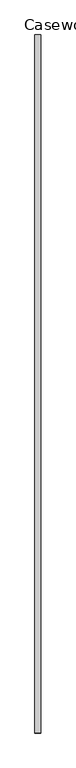
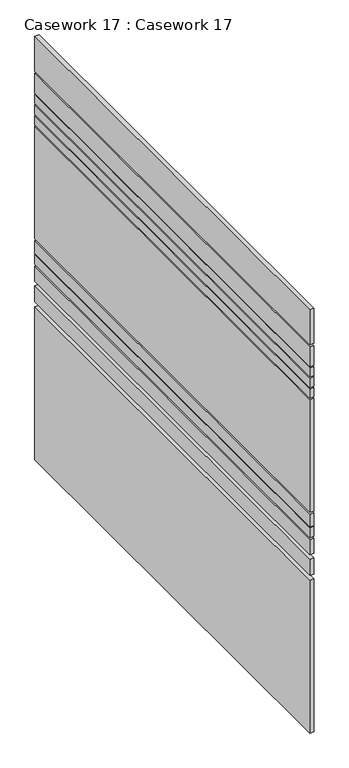
"""IFC4 building model written with IfcOpenShell, lengths in millimetres: furniture geometry, Casework 17 : Casework 17."""

from ifc_helpers import new_model, si_unit, frame, origin, place, context, project, spatial, polyline, outline, extrude, source, transform, mapped, element, save


def casework_17_casework_17_3fc012a0(model_context):
    return source(origin(), model_context, "Body", "SweptSolid", [
        extrude(outline(polyline([(14425.1923267, 11676.4496924), (14425.1923267, 8730.0496924), (14399.7923267, 8730.0496924), (14399.7923267, 11676.4496924), (14425.1923267, 11676.4496924)])), frame((0.0, 0.0, 3178.4304543), z_axis=(0.0, 0.0, 1.0), x_axis=(1.0, 0.0, 0.0)), (0.0, 0.0, 1.0), 228.6),
        extrude(outline(polyline([(14425.1923267, 11676.4496924), (14425.1923267, 8730.0496924), (14399.7923267, 8730.0496924), (14399.7923267, 11676.4496924), (14425.1923267, 11676.4496924)])), frame((0.0, 0.0, 3035.5068643), z_axis=(0.0, 0.0, 1.0), x_axis=(1.0, 0.0, 0.0)), (0.0, 0.0, 1.0), 128.91865),
        extrude(outline(polyline([(14425.1923267, 11676.4496924), (14425.1923267, 8730.0496924), (14399.7923267, 8730.0496924), (14399.7923267, 11676.4496924), (14425.1923267, 11676.4496924)])), frame((0.0, 0.0, 2968.7810931), z_axis=(0.0, 0.0, 1.0), x_axis=(1.0, 0.0, 0.0)), (0.0, 0.0, 1.0), 58.7193149),
        extrude(outline(polyline([(14425.1923267, 11676.4496924), (14425.1923267, 8730.0496924), (14399.7923267, 8730.0496924), (14399.7923267, 11676.4496924), (14425.1923267, 11676.4496924)])), frame((0.0, 0.0, 2897.7011025), z_axis=(0.0, 0.0, 1.0), x_axis=(1.0, 0.0, 0.0)), (0.0, 0.0, 1.0), 63.4634281),
        extrude(outline(polyline([(14425.1923267, 11676.4496924), (14425.1923267, 8730.0496924), (14399.7923267, 8730.0496924), (14399.7923267, 11676.4496924), (14425.1923267, 11676.4496924)])), frame((0.0, 0.0, 2828.852965), z_axis=(0.0, 0.0, 1.0), x_axis=(1.0, 0.0, 0.0)), (0.0, 0.0, 1.0), 58.9081284),
        extrude(outline(polyline([(14425.1923267, 11676.4496924), (14425.1923267, 8730.0496924), (14399.7923267, 8730.0496924), (14399.7923267, 11676.4496924), (14425.1923267, 11676.4496924)])), frame((0.0, 0.0, 2083.8020688), z_axis=(0.0, 0.0, 1.0), x_axis=(1.0, 0.0, 0.0)), (0.0, 0.0, 1.0), 736.5726112),
        extrude(outline(polyline([(14425.1923267, 11676.4496924), (14425.1923267, 8730.0496924), (14399.7923267, 8730.0496924), (14399.7923267, 11676.4496924), (14425.1923267, 11676.4496924)])), frame((0.0, 0.0, 1989.1412316), z_axis=(0.0, 0.0, 1.0), x_axis=(1.0, 0.0, 0.0)), (0.0, 0.0, 1.0), 83.5151082),
        extrude(outline(polyline([(14425.1923267, 11676.4496924), (14425.1923267, 8730.0496924), (14399.7923267, 8730.0496924), (14399.7923267, 11676.4496924), (14425.1923267, 11676.4496924)])), frame((0.0, 0.0, 1917.9922119), z_axis=(0.0, 0.0, 1.0), x_axis=(1.0, 0.0, 0.0)), (0.0, 0.0, 1.0), 66.4625968),
        extrude(outline(polyline([(14425.1923267, 11676.4496924), (14425.1923267, 8730.0496924), (14399.7923267, 8730.0496924), (14399.7923267, 11676.4496924), (14425.1923267, 11676.4496924)])), frame((0.0, 0.0, 1808.3191542), z_axis=(0.0, 0.0, 1.0), x_axis=(1.0, 0.0, 0.0)), (0.0, 0.0, 1.0), 96.6808458),
        extrude(outline(polyline([(14425.1923267, 11676.4496924), (14425.1923267, 8730.0496924), (14399.7923267, 8730.0496924), (14399.7923267, 11676.4496924), (14425.1923267, 11676.4496924)])), frame((0.0, 0.0, 1672.3811779), z_axis=(0.0, 0.0, 1.0), x_axis=(1.0, 0.0, 0.0)), (0.0, 0.0, 1.0), 106.6182975),
        extrude(outline(polyline([(14425.1923267, 11676.4496924), (14425.1923267, 8730.0496924), (14399.7923267, 8730.0496924), (14399.7923267, 11676.4496924), (14425.1923267, 11676.4496924)])), frame((0.0, 0.0, 642.3414243), z_axis=(0.0, 0.0, 1.0), x_axis=(1.0, 0.0, 0.0)), (0.0, 0.0, 1.0), 999.6450066),
    ])


if __name__ == "__main__":
    model = new_model("IFC4")
    model_context = context("Model", 3, world=origin())
    ifc_project = project(units=[si_unit("LENGTHUNIT", "METRE", prefix="MILLI")], contexts=[model_context])
    site = spatial("IfcSite", under=ifc_project)
    building = spatial("IfcBuilding", under=site)
    placement = place(None, origin())
    casework_17_casework_17_shape = casework_17_casework_17_3fc012a0(model_context)
    element("IfcFurniture", 1, ObjectType="Casework 17 : Casework 17", at=placement, inside=building, context=model_context, shape_type="MappedRepresentation", body=[
        mapped(casework_17_casework_17_shape, transform((0.0, 0.0, 0.0), x_axis=(1.0, 0.0, 0.0), y_axis=(0.0, 1.0, 0.0), z_axis=(0.0, 0.0, 1.0))),
    ])
    save(model, "model.ifc")
